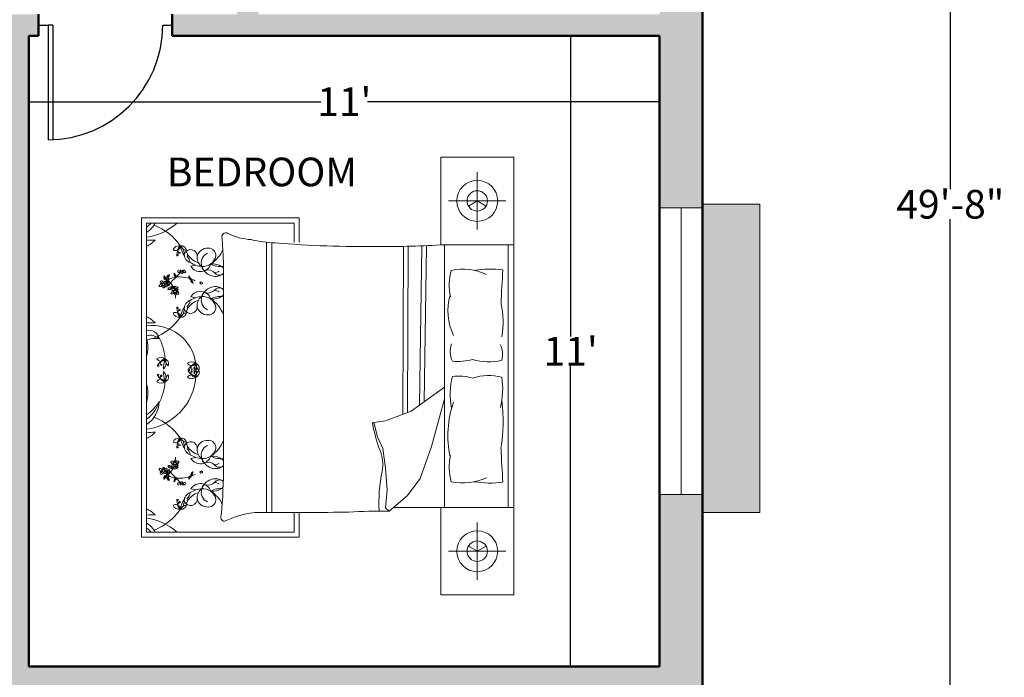
# Model space of a CAD drawing. Units: inches. Extents: x -28 to 544, y -640 to 52.
# Tile 9 of 11: x 338 to 544, y -389 to -251. Entities that reach past the tile are written whole.
import ezdxf

# ---------------------------------------------------------------- set-up
doc = ezdxf.new("R2010")
doc.units = ezdxf.units.IN
doc.header["$MEASUREMENT"] = 0
for name, color, linetype, lineweight in [('A-ANNO-DIMS', 2, 'Continuous', 18), ('A-AREA-IDEN', 7, 'Continuous', 25), ('A-DOOR', 3, 'Continuous', 25), ('A-FURN', 8, 'Continuous', 18), ('A-GLAZ', 4, 'Continuous', 20), ('A-ROOF', 8, 'Continuous', 18), ('A-ROOF-PATT', 252, 'Continuous', 13), ('A-WALL', 7, 'Continuous', 50), ('A-WALL-PATT', 5, 'Continuous', 13)]:
    doc.layers.add(name, color=color, linetype=linetype, lineweight=lineweight)
doc.styles.get("Standard").update_dxf_attribs({"font": 'arial.ttf'})
doc.dimstyles.get("Standard").update_dxf_attribs({"dimtxt": 0.18, "dimasz": 0.18, "dimexe": 0.18, "dimexo": 0.0625, "dimgap": 0.09, "dimtad": 0, "dimtih": 1, "dimtoh": 1, "dimdec": 0, "dimzin": 0, "dimdsep": 46, "dimlunit": 3, "dimtxsty": 'Standard', "dimcen": 0.09, "dimadec": 0, "dimazin": 0, "dimtfac": 1, "dimtdec": 0, "dimtofl": 0, "dimtmove": 0, "dimatfit": 3, "dimfxl": 1, "dimtolj": 1, "dimtzin": 0, "dimarcsym": 0})

# ---------------------------------------------------------------- blocks, each defined once
blk = doc.blocks.new('*D19')
at = {"layer": 'A-ANNO-DIMS', "color": 0, "lineweight": -2, "transparency": 16777216}
for p, q in [((339.44, -274.72), (339.44, -268.35)), ((339.62, -268.53), (400.55, -268.53)), ((471.26, -268.53), (410.34, -268.53)), ((471.44, -274.72), (471.44, -268.35))]:
    blk.add_line(p, q, dxfattribs=at)
at = {"layer": 'A-ANNO-DIMS', "color": 0, "transparency": 16777216}
for points in [[(339.62, -268.5), (339.62, -268.56), (339.44, -268.53)], [(471.26, -268.5), (471.26, -268.56), (471.44, -268.53)]]:
    blk.add_solid(points, dxfattribs=at)
at = {"layer": 'Defpoints', "color": 0, "transparency": 16777216}
for p in [(471.44, -268.53), (339.44, -274.78), (471.44, -274.78)]:
    blk.add_point(p, dxfattribs=at)
at = {"layer": 'A-ANNO-DIMS', "color": 0, "transparency": 16777216, "insert": (405.44, -268.53), "char_height": 6, "attachment_point": 5}
blk.add_mtext("\\A1;11'", dxfattribs=at)
blk = doc.blocks.new('*D20')
at = {"layer": 'A-ANNO-DIMS', "color": 0, "lineweight": -2, "transparency": 16777216}
for p, q in [((452.83, -254.92), (452.83, -317.64)), ((452.89, -254.74), (453.01, -254.74)), ((452.83, -386.56), (452.83, -323.84)), ((452.89, -386.74), (453.01, -386.74))]:
    blk.add_line(p, q, dxfattribs=at)
at = {"layer": 'A-ANNO-DIMS', "color": 0, "transparency": 16777216}
for points in [[(452.8, -254.92), (452.86, -254.92), (452.83, -254.74)], [(452.8, -386.56), (452.86, -386.56), (452.83, -386.74)]]:
    blk.add_solid(points, dxfattribs=at)
at = {"layer": 'Defpoints', "color": 0, "transparency": 16777216}
for p in [(452.83, -254.74), (452.83, -386.74), (452.83, -386.74)]:
    blk.add_point(p, dxfattribs=at)
at = {"layer": 'A-ANNO-DIMS', "color": 0, "transparency": 16777216, "insert": (452.83, -320.74), "char_height": 6, "attachment_point": 5}
blk.add_mtext("\\A1;11'", dxfattribs=at)
blk = doc.blocks.new('*D28')
at = {"layer": 'A-ANNO-DIMS', "color": 0, "lineweight": -2, "transparency": 16777216}
for p, q in [((480.51, 7.76), (532.47, 7.76)), ((532.29, 7.58), (532.29, -286.84)), ((532.29, -587.56), (532.29, -293.14)), ((480.51, -587.74), (532.47, -587.74))]:
    blk.add_line(p, q, dxfattribs=at)
at = {"layer": 'A-ANNO-DIMS', "color": 0, "transparency": 16777216}
for points in [[(532.26, 7.58), (532.32, 7.58), (532.29, 7.76)], [(532.26, -587.56), (532.32, -587.56), (532.29, -587.74)]]:
    blk.add_solid(points, dxfattribs=at)
at = {"layer": 'Defpoints', "color": 0, "transparency": 16777216}
for p in [(480.44, 7.76), (480.44, -587.74), (532.29, -587.74)]:
    blk.add_point(p, dxfattribs=at)
at = {"layer": 'A-ANNO-DIMS', "color": 0, "transparency": 16777216, "insert": (532.29, -289.99), "char_height": 6, "attachment_point": 5}
blk.add_mtext('\\A1;49\'-8"', dxfattribs=at)
blk = doc.blocks.new('BED-DOUBLE-HEADBOARD-92')
for p, q in [((77.93, 0), (77.93, 91.63)), ((70.29, 76.48), (70.29, 88.45)), ((64.3, 82.47), (76.28, 82.47)), ((0, 78.9), (0, 12.09)), ((33.01, 78.9), (0, 78.9)), ((33.01, 73.82), (33.01, 78.9)), ((1.06, 77.84), (31.95, 77.84)), ((1.06, 13.16), (1.06, 77.84)), ((31.95, 77.84), (31.95, 73.8)), ((26.15, 73.81), (26.15, 17.27)), ((27.29, 73.72), (27.29, 17.27)), ((54.87, 72.98), (54.73, 37.82)), ((55.81, 72.98), (55.68, 38.18)), ((58.7, 73.02), (58.23, 39.75)), ((59.64, 73.06), (59.18, 40.44)), ((63.45, 18.33), (63.45, 73.3)), ((76.75, 73.3), (76.75, 18.33)), ((10.35, 68.81), (11.39, 69.01)), ((17.15, 64.42), (17.15, 27.21)), ((10.35, 62.4), (11.39, 62.2)), ((63.45, 43.5), (56.46, 38.48)), ((60.72, 31.05), (63.45, 41.05)), ((56.46, 38.48), (51.08, 36.44)), ((51.08, 36.44), (48.67, 36.07)), ((48.67, 36.07), (49.41, 33.1)), ((49.41, 33.1), (50.52, 30.68)), ((58.31, 24.37), (60.72, 31.05)), ((50.52, 30.68), (51.08, 26.6)), ((10.35, 28.59), (11.39, 28.79)), ((51.08, 26.6), (51.45, 21.96)), ((55.71, 20.85), (58.31, 24.37)), ((10.35, 22.19), (11.39, 21.98)), ((51.45, 21.96), (51.08, 18.25)), ((51.82, 17.51), (55.71, 20.85)), ((31.95, 17.28), (31.95, 13.16)), ((33.01, 12.09), (33.01, 17.28)), ((51.08, 18.25), (51.82, 17.51)), ((77.93, 18.33), (52.78, 18.33)), ((70.29, 15.15), (70.29, 3.18)), ((31.95, 13.16), (1.06, 13.16)), ((0, 12.09), (33.01, 12.09)), ((64.3, 9.16), (76.28, 9.16))]:
    blk.add_line(p, q)
for points in [[(77.93, 73.3), (62.65, 73.3), (62.65, 91.63), (77.93, 91.63)], [(70.29, 82.47), (68.44, 81.4)], [(70.29, 82.47), (72.14, 81.4)], [(62.65, 18.33), (62.65, 0), (77.93, 0)], [(70.29, 9.16), (68.44, 10.23)], [(70.29, 9.16), (72.14, 10.23)]]:
    blk.add_lwpolyline(points)
for points in [[(28.01, 73.7, -0.056112), (22.97, 74.36, -0.095341), (18.12, 75.65)], [(75.64, 68.04, 0.074897), (69.66, 67.93, -0.472817)], [(69.32, 49.3, 0.14099), (75.43, 49.12, 0.235245)], [(69.32, 45.39, -0.14099), (75.43, 45.57, -0.235245)], [(75.64, 23.59, -0.074897), (69.66, 23.7, 0.472817)], [(43.43, 17.31, -0.001242), (26.04, 17.27, 0.127202), (17.38, 15.43)]]:
    blk.add_lwpolyline(points, format="xyb")
for centre, radius in [((70.29, 82.47), 4.28), ((70.29, 82.47), 2.14), ((4.57, 65.04), 0.233), ((7.03, 63.51), 0.233), ((7.03, 27.48), 0.233), ((4.57, 25.95), 0.233), ((70.29, 9.16), 4.28), ((70.29, 9.16), 2.14)]:
    blk.add_circle(centre, radius)
for centre, radius, start, end in [((-2.15, 80.74), 5.83, 303.4617, 330.1116), ((-3.24, 82.84), 7.27, 306.3036, 316.4814), ((-0.55, 86.74), 11.97, 277.745, 311.8856), ((-1.73, 66.27), 11.97, 34.3865, 68.5908), ((-0.8, 77.48), 4.87, 292.5547, 318.9546), ((1.81, 90.8), 16.56, 267.4081, 273.6519), ((17.65, 74.95), 0.835, 56.1736, 203.4781), ((-71.97, 67.22), 89.16, 358.1965, 4.7598), ((7.86, 71.73), 1.33, 77.7115, 159.0387), ((7.14, 73.06), 0.999, 238.4633, 358.2869), ((10.42, 71.04), 3.03, 138.8402, 177.9352), ((8.6, 72.16), 0.979, 117.6827, 223.7762), ((8.38, 72.07), 0.992, 2.9516, 103.728), ((16.31, 74.84), 8.37, 192.5173, 207.1824), ((7.04, 71.5), 1.89, 345.4653, 54.2343), ((9.89, 74.09), 2.04, 211.3827, 255.2969), ((10.28, 70.9), 1.38, 350.264, 160.8688), ((13.81, 70.4), 2.19, 84.9449, 172.8857), ((14.03, 71.03), 1.55, 354.4856, 91.0538), ((10.7, 75.07), 6.94, 303.6671, 336.3547), ((46.26, 287.69), 214.77, 265.1265, 270.8855), ((52.25, 237.57), 164.64, 269.0718, 273.9), ((7.54, 71.14), 0.149, 177.9352, 11.4834), ((7.62, 71.16), 0.0722, 11.4834, 127.9409), ((8.03, 71.59), 0.078, 223.7729, 159.7333), ((10.69, 71.23), 1.72, 175.969, 254.3045), ((8.79, 71.18), 0.843, 333.9755, 53.2681), ((8.41, 69.38), 1.83, 6.1662, 51.5825), ((13.3, 73.63), 4.33, 211.2614, 251.7045), ((14.29, 70.78), 2.66, 182.3591, 234.0401), ((14.64, 69.54), 2.13, 111.5819, 201.4221), ((12.88, 71.51), 2.76, 265.2933, 346.921), ((7.99, 67.72), 0.385, 127.7621, 169.0403), ((8.42, 68.04), 0.233, 183.2768, 356.7232), ((8.78, 67.71), 0.389, 11.5637, 52.6358), ((12.96, 73.67), 4.92, 236.2883, 266.5076), ((12.33, 69.94), 2.28, 209.9085, 343.1337), ((13.28, 68.5), 0.569, 167.3041, 285.1471), ((14.82, 65.78), 3.53, 122.7011, 126.3445), ((15.49, 69.59), 2.92, 199.2822, 299.1751), ((13.92, 66.14), 1.88, 41.5653, 105.1471), ((16.47, 72.53), 3.8, 238.8218, 280.751), ((14.82, 65.78), 3.53, 55.785, 94.7304), ((16.14, 67.83), 1.1, 17.4186, 52.325), ((67.25, 56.37), 11.81, 65.1316, 101.7583), ((947.66, 17.54), 873.48, 176.68521, 177.14978), ((4.91, 66.54), 0.261, 124.3538, 214.3923), ((5.29, 66.5), 0.608, 190.3057, 287.1958), ((5.47, 66.72), 0.705, 176.9701, 248.2913), ((10.5, 70.44), 6.82, 212.6784, 216.3746), ((5.23, 66.56), 0.27, 216.3746, 291.7548), ((3.7, 62.29), 4.06, 63.7819, 68.2913), ((5.88, 66.37), 0.608, 122.8155, 187.3992), ((5.41, 66.12), 0.204, 289.3605, 111.7548), ((5.56, 66.12), 0.204, 221.8703, 44.2646), ((6.14, 66.29), 0.705, 109.4799, 177.6828), ((5.76, 66.74), 0.261, 56.8636, 146.9021), ((5.9, 66.45), 0.27, 148.8844, 224.2646), ((11.5, 63.06), 6.82, 145.1882, 148.8844), ((7.62, 62.77), 3.8, 94.756, 119.2041), ((15.72, 57.29), 12.52, 132.2412, 142.1744), ((9.4, 67.26), 2.58, 178.3264, 187.1302), ((6.61, 66.9), 0.481, 11.3256, 64.4621), ((8.24, 67.59), 1.45, 190.2588, 210.656), ((7.27, 67), 0.44, 188.3432, 274.2869), ((7.66, 67.24), 0.768, 210.656, 242.6341), ((8.24, 67.9), 1.47, 218.2101, 226.3071), ((7.15, 66.67), 0.187, 325.7657, 67.4417), ((1.35, 72.91), 8.7, 313.1541, 322.0459), ((7.81, 58.99), 7.59, 73.5842, 93.8277), ((7.75, 67.68), 0.179, 142.4737, 265.053), ((7.78, 68.04), 0.542, 265.053, 338.3618), ((8.5, 67.3), 0.709, 113.4276, 137.6104), ((8.59, 67.61), 0.382, 139.7889, 227.6792), ((8.47, 67.48), 0.201, 227.6792, 350.3487), ((7.69, 67.62), 0.764, 353.0852, 15.7171), ((8.19, 67.53), 0.482, 350.3487, 43.6538), ((9.08, 68.03), 0.561, 198.7263, 262.5032), ((8.64, 67.76), 0.223, 1.1081, 91.8675), ((9.06, 67.64), 0.18, 255.2356, 54.9248), ((12.48, 66.71), 2.58, 178.3264, 187.1302), ((9.69, 66.35), 0.481, 11.3256, 64.4621), ((11.32, 67.04), 1.45, 190.2588, 210.656), ((10.35, 66.45), 0.44, 188.3432, 274.2869), ((10.74, 66.7), 0.768, 210.656, 242.6341), ((11.32, 67.36), 1.47, 218.2101, 226.3071), ((10.23, 66.12), 0.187, 325.7657, 67.4417), ((10.76, 65.78), 0.44, 147.5332, 233.4768), ((11.15, 66), 0.768, 179.1859, 211.164), ((10.41, 65.83), 0.187, 354.3784, 96.0543), ((7.81, 58.99), 7.59, 63.0032, 69.8941), ((14.96, 70.03), 2.63, 277.436, 299.9149), ((16.35, 68.29), 1.37, 221.5653, 293.8354), ((16.14, 67.83), 1.1, 314.4517, 343.3657), ((76.71, 64.77), 12.28, 165.1039, 191.0369), ((3.9, 64.68), 0.179, 142.4737, 265.053), ((4.14, 64.72), 0.385, 61.2196, 169.0403), ((3.93, 65.05), 0.542, 265.053, 338.3618), ((4.39, 65.51), 0.461, 157.4086, 261.4386), ((4.13, 65.53), 0.231, 58.0499, 135.6268), ((4.65, 64.3), 0.709, 113.4276, 137.6104), ((4.37, 65.38), 0.155, 172.906, 277.132), ((3.87, 65.1), 0.736, 14.7558, 58.0499), ((4.74, 64.62), 0.382, 139.7889, 227.6792), ((4.62, 64.48), 0.201, 227.6792, 350.3487), ((4.9, 65.3), 0.318, 36.1046, 181.4281), ((3.84, 64.62), 0.764, 353.0852, 15.7171), ((4.34, 64.53), 0.482, 350.3487, 43.6538), ((4.71, 65.55), 0.321, 270.0645, 331.1507), ((4.98, 65.47), 0.367, 221.8413, 265.7877), ((5.24, 65.03), 0.561, 198.7263, 262.5032), ((4.79, 64.77), 0.223, 1.1081, 91.8675), ((4.98, 65.33), 0.229, 263.7526, 41.7054), ((4.93, 64.72), 0.389, 11.5637, 86.365), ((7.62, 62.77), 3.8, 124.0033, 132.4917), ((5.21, 64.65), 0.18, 255.2356, 54.9248), ((5.88, 65.42), 0.647, 128.3208, 208.8162), ((5.99, 65.47), 0.773, 207.7043, 254.3516), ((6.48, 65.52), 1.06, 157.2305, 229.0635), ((5.49, 65.02), 1.06, 270.278, 342.111), ((6.2, 63.69), 0.752, 98.7227, 159.3375), ((5.82, 64.66), 0.773, 244.9899, 291.6373), ((6.12, 65.88), 0.626, 174.4544, 220.6188), ((2.56, 62.38), 4.56, 30.544, 49.818), ((5.08, 64.98), 0.752, 340.0041, 40.6188), ((5.99, 65.06), 0.626, 278.7227, 324.8872), ((5.88, 64.55), 0.647, 290.5253, 358.5375), ((6.85, 63.99), 0.461, 157.4086, 261.4386), ((6.59, 64), 0.231, 58.0499, 135.6268), ((7.14, 64.73), 0.647, 182.8499, 266.1226), ((6.89, 65.19), 0.626, 231.7607, 277.9252), ((7.38, 65.3), 1.06, 214.5369, 286.3699), ((6.33, 63.57), 0.736, 14.7558, 58.0499), ((2.56, 62.38), 4.56, 23.0501, 23.8477), ((7.08, 63.82), 0.752, 37.3105, 97.9252), ((7.36, 63.77), 0.318, 36.1046, 181.4281), ((7.16, 64.86), 0.773, 265.0106, 311.658), ((7.44, 63.81), 0.229, 263.7526, 41.7054), ((11.99, 67.54), 2.58, 234.6898, 243.4936), ((11.74, 66.36), 1.45, 211.164, 231.5612), ((12.01, 66.21), 1.47, 195.5129, 203.6099), ((10.35, 65.24), 0.481, 357.3579, 50.4944), ((12.42, 65.34), 0.177, 12.7051, 190.4384), ((12.53, 65.36), 0.287, 190.4384, 10.4136), ((15.49, 61.62), 2.92, 60.8249, 160.7178), ((16.35, 62.91), 1.37, 66.1646, 138.4347), ((16.14, 63.38), 1.1, 23.2856, 45.5483), ((6.36, 63.16), 0.179, 142.4737, 265.053), ((6.6, 63.19), 0.385, 61.2196, 169.0403), ((6.39, 63.52), 0.542, 265.053, 338.3618), ((7.11, 62.78), 0.709, 113.4276, 137.6104), ((6.83, 63.86), 0.155, 172.906, 277.132), ((7.2, 63.09), 0.382, 139.7889, 227.6792), ((7.08, 62.96), 0.201, 227.6792, 350.3487), ((6.3, 63.09), 0.764, 353.0852, 15.7171), ((2.56, 62.38), 4.56, 357.1071, 4.7585), ((6.8, 63), 0.482, 350.3487, 43.6538), ((7.17, 64.02), 0.321, 270.0645, 331.1507), ((7.44, 63.94), 0.367, 221.8413, 265.7877), ((7.7, 63.5), 0.561, 198.7263, 262.5032), ((7.25, 63.24), 0.223, 1.1081, 91.8675), ((7.39, 63.19), 0.389, 11.5637, 86.365), ((7.67, 63.12), 0.18, 255.2356, 54.9248), ((12.96, 57.54), 4.92, 93.4924, 123.7117), ((12.33, 61.27), 2.28, 16.8663, 150.0915), ((14.29, 60.43), 2.66, 125.9599, 177.6409), ((14.64, 61.67), 2.13, 158.5779, 248.4181), ((12.88, 59.7), 2.76, 13.079, 94.7067), ((13.28, 62.71), 0.569, 74.8529, 192.6959), ((14.82, 65.43), 3.53, 233.6555, 237.2989), ((13.92, 65.07), 1.88, 254.8529, 318.4347), ((16.47, 58.68), 3.8, 79.7133, 121.1782), ((14.82, 65.43), 3.53, 265.2696, 304.215), ((10.7, 56.14), 6.94, 21.4941, 56.3329), ((14.96, 61.18), 2.63, 60.0851, 82.564), ((16.14, 63.38), 1.1, 307.675, 336.7144), ((75.81, 59.47), 11.66, 163.8254, 206.1239), ((7.54, 60.07), 0.149, 348.5166, 182.0648), ((10.42, 60.17), 3.03, 182.0648, 221.1598), ((7.62, 60.05), 0.0722, 232.0591, 348.5166), ((7.04, 59.71), 1.89, 305.7657, 14.5347), ((16.31, 56.36), 8.37, 152.8176, 167.4827), ((10.69, 59.98), 1.72, 105.6955, 184.031), ((10.28, 60.31), 1.38, 199.1312, 9.736), ((8.79, 60.02), 0.843, 306.7319, 26.0245), ((8.41, 61.83), 1.83, 308.4175, 353.8338), ((13.3, 57.58), 4.33, 108.2955, 148.7386), ((13.81, 60.81), 2.19, 187.1143, 275.0551), ((14.03, 60.18), 1.55, 268.9462, 5.5144), ((59.61, 57.17), 16.11, 348.8159, 13.6573), ((-0.8, 53.73), 4.87, 41.0454, 67.4453), ((-1.73, 64.94), 11.97, 291.4092, 325.6135), ((7.14, 58.15), 0.999, 1.7131, 121.5367), ((7.86, 59.47), 1.33, 200.9613, 282.2885), ((8.6, 59.04), 0.979, 136.2238, 242.3173), ((7.98, 59.63), 0.129, 200.2817, 136.2238), ((8.38, 59.14), 0.992, 256.272, 357.0484), ((9.89, 57.11), 2.04, 104.7031, 148.6173), ((1.81, 40.41), 16.56, 86.3481, 92.5919), ((2.21, 47.13), 9.26, 8.1803, 97.1364), ((1.57, 53.24), 2.15, 10.9261, 103.6102), ((1.86, 51.63), 2.72, 48.0951, 107.1391), ((-5.23, 51.78), 6.58, 343.5431, 17.0202), ((3.06, 48.33), 5.36, 83.3805, 111.883), ((-6.96, 48.43), 11.97, 4.4623, 27.4146), ((69.49, 50.99), 4.86, 161.4593, 204.9817), ((71.07, 50.37), 4.53, 343.8974, 26.6563), ((-8.62, 49.17), 9.73, 4.3787, 5.6357), ((-15.29, 44.05), 17.39, 19.7217, 19.9028), ((4.08, 48.38), 1.33, 47.7873, 129.1145), ((4.12, 49.89), 0.999, 208.5391, 328.3627), ((3.51, 48.03), 0.149, 148.011, 341.5592), ((5.95, 46.5), 3.03, 108.9159, 148.011), ((3.58, 48), 0.0722, 341.5592, 98.0167), ((4.93, 48.39), 0.979, 87.7585, 193.852), ((4.16, 48.17), 0.078, 193.9791, 129.8091), ((12.96, 46.86), 8.37, 162.593, 177.2582), ((3.25, 48.59), 1.89, 315.5411, 24.3101), ((7.01, 49.42), 2.04, 181.4585, 225.3727), ((4.69, 48.41), 0.992, 333.0274, 73.8037), ((10.49, 47.47), 1.33, 47.7873, 129.1145), ((10.53, 48.97), 0.999, 208.5391, 328.3627), ((12.36, 45.59), 3.03, 108.9159, 148.011), ((11.34, 47.47), 0.979, 87.7585, 193.852), ((9.65, 47.67), 1.89, 315.5411, 24.3101), ((19.37, 45.95), 8.37, 162.593, 177.2582), ((9.65, 46.38), 1.89, 335.6899, 44.4589), ((19.37, 48.1), 8.37, 182.7418, 197.407), ((11.1, 47.5), 0.992, 333.0274, 73.8037), ((13.42, 48.5), 2.04, 181.4585, 225.3727), ((66.26, 60.1), 11.23, 264.0129, 285.8293), ((-0.55, 46.53), 11.97, 277.745, 355.5377), ((3.51, 46.02), 0.149, 18.4408, 211.989), ((5.95, 47.54), 3.03, 211.989, 251.0841), ((3.58, 46.04), 0.0722, 261.9833, 18.4408), ((4.93, 45.66), 0.979, 166.148, 272.2415), ((4.11, 45.86), 0.129, 230.0755, 166.148), ((12.96, 47.19), 8.37, 182.7418, 197.407), ((3.25, 45.46), 1.89, 335.6899, 44.4589), ((7.01, 44.63), 2.04, 134.6273, 178.5415), ((4.69, 45.63), 0.992, 286.1963, 26.9726), ((10.53, 45.07), 0.999, 31.6373, 151.4609), ((10.49, 46.58), 1.33, 230.8855, 312.2127), ((9.92, 47.11), 0.149, 148.011, 341.5592), ((9.92, 46.94), 0.149, 18.4408, 211.989), ((12.36, 48.46), 3.03, 211.989, 251.0841), ((9.99, 47.09), 0.0722, 341.5592, 98.0167), ((9.99, 46.96), 0.0722, 261.9833, 18.4408), ((11.34, 46.58), 0.979, 166.148, 272.2415), ((10.52, 46.78), 0.129, 230.0755, 166.148), ((10.57, 47.26), 0.078, 193.9791, 129.8091), ((11.1, 46.55), 0.992, 286.1963, 26.9726), ((13.42, 45.55), 2.04, 134.6273, 178.5415), ((80.79, 41.94), 16.16, 166.3762, 190.1383), ((66.26, 34.58), 11.23, 74.1707, 95.9871), ((59.28, 43.16), 16.33, 346.04, 8.4751), ((-5.23, 42.27), 6.58, 342.9798, 16.4569), ((-8.62, 44.87), 9.73, 354.3643, 355.6213), ((-15.29, 50), 17.39, 340.0972, 340.2783), ((4.12, 44.16), 0.999, 31.6373, 151.4609), ((4.08, 45.66), 1.33, 230.8855, 312.2127), ((-6.96, 45.61), 11.97, 332.5854, 355.5377), ((-2.15, 40.53), 5.83, 303.4617, 358.728), ((-5.28, 46.44), 10.81, 305.947, 325.9877), ((-3.24, 42.62), 7.27, 306.3036, 342.1496), ((85.44, 33.32), 21.3, 160.7385, 191.9603), ((42.48, 36.14), 33.23, 350.503, 7.7804), ((-1.73, 26.06), 11.97, 34.3865, 68.5908), ((48.59, 35.86), 0.221, 70.2464, 181.1377), ((83.29, 42.43), 35.54, 190.6617, 199.8806), ((1.81, 50.59), 16.56, 267.4081, 273.6519), ((-0.8, 37.26), 4.87, 292.5547, 318.9546), ((7.86, 31.52), 1.33, 77.7115, 159.0387), ((7.14, 32.84), 0.999, 238.4633, 358.2869), ((7.54, 30.93), 0.149, 177.9352, 11.4834), ((10.42, 30.82), 3.03, 138.8402, 177.9352), ((7.62, 30.94), 0.0722, 11.4834, 127.9409), ((8.6, 31.95), 0.979, 117.6827, 223.7762), ((8.03, 31.37), 0.078, 223.7729, 159.7333), ((8.38, 31.85), 0.992, 2.9516, 103.728), ((9.89, 33.88), 2.04, 211.3827, 255.2969), ((7.04, 31.28), 1.89, 345.4653, 54.2343), ((16.31, 34.63), 8.37, 192.5173, 207.1824), ((10.69, 31.02), 1.72, 175.969, 254.3045), ((10.28, 30.69), 1.38, 350.264, 160.8688), ((8.79, 30.97), 0.843, 333.9755, 53.2681), ((13.3, 33.41), 4.33, 211.2614, 251.7045), ((13.81, 30.18), 2.19, 84.9449, 172.8857), ((14.64, 29.32), 2.13, 111.5819, 201.4221), ((14.03, 30.82), 1.55, 354.4856, 91.0538), ((10.7, 34.86), 6.94, 303.6671, 338.5059), ((8.41, 29.17), 1.83, 6.1662, 51.5825), ((12.96, 33.45), 4.92, 236.2883, 266.5076), ((12.33, 29.73), 2.28, 209.9085, 343.1337), ((14.29, 30.56), 2.66, 182.3591, 234.0401), ((12.88, 31.29), 2.76, 265.2933, 346.921), ((16.47, 32.31), 3.8, 238.8218, 280.2867), ((14.82, 25.56), 3.53, 55.785, 94.7304), ((43.05, 27.34), 7.46, 348.6608, 23.7384), ((76.71, 26.86), 12.28, 168.9631, 194.8961), ((947.66, 74.1), 873.48, 182.85022, 183.31479), ((5.82, 26.33), 0.773, 68.3627, 115.0101), ((5.49, 25.97), 1.06, 17.889, 89.722), ((6.2, 27.3), 0.752, 200.6625, 261.2773), ((5.88, 26.45), 0.647, 1.4625, 69.4747), ((6.36, 27.83), 0.179, 94.947, 217.5263), ((6.6, 27.8), 0.385, 190.9597, 298.7804), ((6.39, 27.47), 0.542, 21.6382, 94.947), ((6.85, 27), 0.461, 98.5614, 202.5914), ((6.59, 26.99), 0.231, 224.3732, 301.9501), ((7.14, 26.26), 0.647, 93.8774, 177.1501), ((7.11, 28.21), 0.709, 222.3896, 246.5724), ((6.83, 27.13), 0.155, 82.868, 187.094), ((6.33, 27.42), 0.736, 301.9501, 345.2442), ((2.56, 28.61), 4.56, 336.1523, 336.9499), ((7.2, 27.9), 0.382, 132.3208, 220.2111), ((7.08, 28.04), 0.201, 9.6513, 132.3208), ((6.3, 27.9), 0.764, 344.2829, 6.9148), ((7.36, 27.22), 0.318, 178.5719, 323.8954), ((7.16, 26.14), 0.773, 48.342, 94.9894), ((2.56, 28.61), 4.56, 355.2415, 2.8929), ((6.8, 27.99), 0.482, 316.3462, 9.6513), ((7.7, 27.49), 0.561, 97.4968, 161.2737), ((7.44, 27.05), 0.367, 94.2123, 138.1587), ((7.17, 26.97), 0.321, 28.8493, 89.9355), ((7.25, 27.75), 0.223, 268.1325, 358.8919), ((7.39, 27.8), 0.389, 273.635, 348.4363), ((7.44, 27.19), 0.229, 318.2946, 96.2474), ((7.67, 27.87), 0.18, 305.0752, 104.7644), ((13.28, 28.28), 0.569, 167.3041, 285.1471), ((14.82, 25.56), 3.53, 122.7011, 126.3445), ((15.49, 29.37), 2.92, 199.2822, 299.1751), ((13.92, 25.92), 1.88, 41.5653, 105.1471), ((14.96, 29.81), 2.63, 277.436, 299.9149), ((16.35, 28.08), 1.37, 221.5653, 293.8354), ((-78.23, 26.12), 95.39, 354.3113, 0.6567), ((16.14, 27.61), 1.1, 23.2856, 52.325), ((16.14, 27.61), 1.1, 314.4517, 336.771), ((3.9, 26.31), 0.179, 94.947, 217.5263), ((4.14, 26.27), 0.385, 190.9597, 298.7804), ((3.93, 25.95), 0.542, 21.6382, 94.947), ((4.39, 25.48), 0.461, 98.5614, 202.5914), ((4.13, 25.46), 0.231, 224.3732, 301.9501), ((4.65, 26.69), 0.709, 222.3896, 246.5724), ((4.37, 25.61), 0.155, 82.868, 187.094), ((3.87, 25.89), 0.736, 301.9501, 345.2442), ((4.74, 26.38), 0.382, 132.3208, 220.2111), ((4.62, 26.51), 0.201, 9.6513, 132.3208), ((3.84, 26.37), 0.764, 344.2829, 6.9148), ((4.9, 25.7), 0.318, 178.5719, 323.8954), ((4.34, 26.46), 0.482, 316.3462, 9.6513), ((5.29, 24.49), 0.608, 72.8042, 169.6943), ((5.24, 25.96), 0.561, 97.4968, 161.2737), ((4.98, 25.52), 0.367, 94.2123, 138.1587), ((4.71, 25.45), 0.321, 28.8493, 89.9355), ((5.47, 24.27), 0.705, 111.7087, 183.0299), ((4.79, 26.23), 0.223, 268.1325, 358.8919), ((4.93, 26.28), 0.389, 273.635, 348.4363), ((4.98, 25.66), 0.229, 318.2946, 96.2474), ((7.62, 28.22), 3.8, 227.5083, 235.9967), ((5.21, 26.35), 0.18, 305.0752, 104.7644), ((3.7, 28.7), 4.06, 291.7087, 296.2181), ((5.88, 25.57), 0.647, 151.1838, 231.6792), ((5.99, 25.53), 0.773, 105.6484, 152.2957), ((5.41, 24.88), 0.204, 248.2452, 70.6395), ((5.56, 24.88), 0.204, 315.7354, 138.1297), ((6.48, 25.47), 1.06, 130.9365, 202.7695), ((6.12, 25.12), 0.626, 139.3812, 185.5456), ((2.56, 28.61), 4.56, 310.182, 329.456), ((5.9, 24.55), 0.27, 135.7354, 211.1156), ((5.08, 26.01), 0.752, 319.3812, 19.9959), ((7.62, 28.22), 3.8, 240.7959, 265.244), ((15.72, 33.7), 12.52, 217.8256, 227.7588), ((5.99, 25.94), 0.626, 35.1128, 81.2773), ((7.38, 25.69), 1.06, 73.6301, 145.4631), ((6.89, 25.81), 0.626, 82.0748, 128.2393), ((7.08, 27.17), 0.752, 262.0748, 322.6895), ((10.35, 24.54), 0.44, 85.7131, 171.6568), ((10.74, 24.29), 0.768, 117.3659, 149.344), ((10.23, 24.87), 0.187, 292.5583, 34.2343), ((10.76, 25.21), 0.44, 126.5232, 212.4668), ((11.15, 24.99), 0.768, 148.836, 180.8141), ((10.41, 25.16), 0.187, 263.9457, 5.6216), ((7.81, 32), 7.59, 290.1059, 296.9968), ((11.99, 23.46), 2.58, 116.5064, 125.3102), ((11.74, 24.64), 1.45, 128.4388, 148.836), ((12.01, 24.79), 1.47, 156.3901, 164.4871), ((10.35, 25.75), 0.481, 309.5056, 2.6421), ((12.42, 25.65), 0.177, 169.5616, 347.2949), ((12.53, 25.63), 0.287, 349.5864, 169.5616), ((84.27, 19.07), 34.58, 168.6608, 182.5481), ((4.91, 24.45), 0.261, 145.6077, 235.6462), ((10.5, 20.55), 6.82, 143.6254, 147.3216), ((5.23, 24.44), 0.27, 68.2452, 143.6254), ((5.88, 24.62), 0.608, 172.6008, 237.1845), ((6.14, 24.7), 0.705, 182.3172, 250.5201), ((5.76, 24.26), 0.261, 213.0979, 303.1364), ((11.5, 27.93), 6.82, 211.1156, 214.8118), ((9.4, 23.73), 2.58, 172.8698, 181.6736), ((8.24, 23.4), 1.45, 149.344, 169.7412), ((6.61, 24.09), 0.481, 295.5379, 348.6744), ((7.27, 23.99), 0.44, 85.7131, 171.6568), ((7.66, 23.75), 0.768, 117.3659, 149.344), ((8.24, 23.09), 1.47, 133.6929, 141.7899), ((7.15, 24.33), 0.187, 292.5583, 34.2343), ((7.81, 32), 7.59, 266.1723, 286.4158), ((1.35, 18.08), 8.7, 37.9541, 46.8459), ((7.75, 23.31), 0.179, 94.947, 217.5263), ((7.99, 23.27), 0.385, 190.9597, 232.2379), ((7.78, 22.95), 0.542, 21.6382, 94.947), ((8.5, 23.69), 0.709, 222.3896, 246.5724), ((8.42, 22.96), 0.233, 3.2768, 176.7232), ((8.59, 23.38), 0.382, 132.3208, 220.2111), ((8.47, 23.51), 0.201, 9.6513, 132.3208), ((7.69, 23.37), 0.764, 344.2829, 6.9148), ((8.19, 23.46), 0.482, 316.3462, 9.6513), ((9.08, 22.97), 0.561, 97.4968, 161.2737), ((8.64, 23.23), 0.223, 268.1325, 358.8919), ((9.06, 23.35), 0.18, 305.0752, 104.7644), ((8.78, 23.28), 0.389, 307.3642, 348.4363), ((11.32, 23.95), 1.45, 149.344, 169.7412), ((12.48, 24.28), 2.58, 172.8698, 181.6736), ((9.69, 24.64), 0.481, 295.5379, 348.6744), ((11.32, 23.63), 1.47, 133.6929, 141.7899), ((12.33, 21.05), 2.28, 16.8663, 150.0915), ((13.28, 22.49), 0.569, 74.8529, 192.6959), ((15.49, 21.4), 2.92, 60.8249, 160.7178), ((13.92, 24.86), 1.88, 254.8529, 318.4347), ((14.96, 20.96), 2.63, 60.0851, 82.564), ((16.35, 22.7), 1.37, 66.1646, 138.4347), ((16.14, 23.17), 1.1, 26.442, 45.5483), ((67.25, 35.26), 11.81, 258.2417, 294.8684), ((10.69, 19.76), 1.72, 105.6955, 184.031), ((8.41, 21.61), 1.83, 308.4175, 353.8338), ((13.3, 17.36), 4.33, 108.2955, 148.7386), ((12.96, 17.32), 4.92, 93.4924, 123.7117), ((14.29, 20.21), 2.66, 125.9599, 177.6409), ((14.64, 21.45), 2.13, 158.5779, 248.4181), ((12.88, 19.48), 2.76, 13.079, 94.7067), ((14.82, 25.21), 3.53, 233.6555, 237.2989), ((16.47, 18.46), 3.8, 80.8446, 121.1782), ((14.82, 25.21), 3.53, 265.2696, 304.215), ((10.7, 15.92), 6.94, 26.7003, 56.3329), ((16.14, 23.17), 1.1, 307.675, 329.9707), ((7.14, 17.93), 0.999, 1.7131, 121.5367), ((7.86, 19.26), 1.33, 200.9613, 282.2885), ((7.54, 19.85), 0.149, 348.5166, 182.0648), ((10.42, 19.95), 3.03, 182.0648, 221.1598), ((7.62, 19.83), 0.0722, 232.0591, 348.5166), ((8.6, 18.83), 0.979, 136.2238, 242.3173), ((7.98, 19.42), 0.129, 200.2817, 136.2238), ((16.31, 16.15), 8.37, 152.8176, 167.4827), ((7.04, 19.5), 1.89, 305.7657, 14.5347), ((9.89, 16.9), 2.04, 104.7031, 148.6173), ((8.38, 18.93), 0.992, 256.272, 357.0484), ((10.28, 20.09), 1.38, 199.1312, 9.736), ((8.79, 19.81), 0.843, 306.7319, 26.0245), ((13.81, 20.59), 2.19, 187.1143, 275.0551), ((14.03, 19.96), 1.55, 268.9462, 5.5144), ((-0.8, 13.52), 4.87, 41.0454, 67.4453), ((1.81, 0.19), 16.56, 86.3481, 92.5919), ((-1.73, 24.72), 11.97, 291.4092, 325.6135), ((17.44, 16.28), 0.845, 152.6588, 266.02), ((49.54, -66.51), 84.05, 88.447, 94.1706), ((-0.55, 4.25), 11.97, 48.1144, 82.255), ((-2.15, 10.25), 5.83, 29.8884, 56.5383), ((-3.24, 8.15), 7.27, 43.5186, 53.6964)]:
    blk.add_arc(centre, radius, start, end)
blk = doc.blocks.new('WIN-60IN')
for p, q in [((0, 9), (60, 9)), ((0, 0), (0, 9)), ((60, 9), (60, 0)), ((0, 4.5), (60, 4.5)), ((60, 0), (0, 0))]:
    blk.add_line(p, q)
blk = doc.blocks.new('DOOR-SWING-24IN')
for p, q in [((25, 0), (25, 24)), ((26, 0), (26, 24)), ((2, 0), (0, 0)), ((25, 0), (26, 0)), ((28, 0), (26, 0))]:
    blk.add_line(p, q)
blk.add_arc((26, 0), 24, 90, 180)

msp = doc.modelspace()

# ---------------------------------------------------------------- hatches: boundary and pattern name
at = {"layer": 'A-ROOF-PATT'}
h = msp.add_hatch(color=256, dxfattribs=at)
h.dxf.hatch_style = 1
h.set_gradient(color1=(241, 235, 31), color2=(248, 153, 30))
h.paths.add_polyline_path([(124.53, 19.76), (58.75, 19.76), (58.75, 7.76), (124.53, 7.76)])
h.paths.add_polyline_path([(226.33, 19.76), (182.83, 19.76), (182.83, 7.76), (226.33, 7.76)])
h.paths.add_polyline_path([(313.67, 19.76), (271.84, 19.76), (271.84, 7.76), (313.67, 7.76)])
h.paths.add_polyline_path([(440.55, 19.76), (372.16, 19.76), (372.16, 7.76), (440.55, 7.76)])
h.paths.add_polyline_path([(492.44, -34.91), (480.44, -34.91), (480.44, -100.18), (492.44, -100.18)])
h.paths.add_polyline_path([(492.44, -151.37), (480.44, -151.37), (480.44, -179.02), (492.44, -179.02)])
h.paths.add_polyline_path([(492.44, -207.96), (480.44, -207.96), (480.44, -238.77), (492.44, -238.77)])
h.paths.add_polyline_path([(492.44, -289.99), (480.44, -289.99), (480.44, -354.53), (492.44, -354.53)])
h.paths.add_polyline_path([(492.44, -399.27), (480.44, -399.27), (480.44, -430), (492.44, -430)])
h.paths.add_polyline_path([(492.44, -475.99), (480.44, -475.99), (480.44, -546.14), (492.44, -546.14)])
h.paths.add_polyline_path([(442.7, -587.74), (368.43, -587.74), (368.43, -599.74), (442.7, -599.74)])
h.paths.add_polyline_path([(127.64, -587.74), (54.75, -587.74), (54.75, -599.74), (127.64, -599.74)])
h.paths.add_polyline_path([(16.94, -477.43), (4.94, -477.43), (4.94, -547.54), (16.94, -547.54)])
h.paths.add_polyline_path([(16.94, -399.8), (4.94, -399.8), (4.94, -430.58), (16.94, -430.58)])
h.paths.add_polyline_path([(16.94, -287.93), (4.94, -287.93), (4.94, -356.82), (16.94, -356.82)])
h.paths.add_polyline_path([(16.94, -208.93), (4.94, -208.93), (4.94, -240.18), (16.94, -240.18)])
h.paths.add_polyline_path([(16.94, -150), (4.94, -150), (4.94, -180.17), (16.94, -180.17)])
h.paths.add_polyline_path([(16.94, -32.89), (4.94, -32.89), (4.94, -101.73), (16.94, -101.73)])
at = {"layer": 'A-WALL-PATT'}
h = msp.add_hatch(color=256, dxfattribs=at)
h.dxf.hatch_style = 1
h.paths.add_polyline_path([(375.44, 7.76), (310.94, 7.76), (310.94, -1.24), (334.94, -1.24), (334.94, -133.24), (286.94, -133.24), (286.94, -137.74), (342.44, -137.74), (342.44, -133.24), (339.44, -133.24), (339.44, -1.24), (375.44, -1.24)])
h.paths.add_polyline_path([(480.44, 7.76), (435.44, 7.76), (435.44, -1.24), (471.44, -1.24), (471.44, -37.24), (480.44, -37.24)])
h.paths.add_polyline_path([(480.44, -97.24), (471.44, -97.24), (471.44, -133.24), (417.44, -133.24), (417.44, -135.49), (417.44, -137.74), (471.44, -137.74), (471.44, -152.74), (480.44, -152.74)])
h.paths.add_polyline_path([(480.44, -176.74), (471.44, -176.74), (471.44, -191.74), (387.44, -191.74), (387.44, -137.74), (389.44, -137.74), (389.44, -133.24), (370.44, -133.24), (370.44, -135.49), (370.44, -137.74), (382.94, -137.74), (382.94, -191.74), (382.94, -196.24), (382.94, -220.24), (385.19, -220.24), (387.44, -220.24), (387.44, -196.24), (471.44, -196.24), (471.44, -211.24), (480.44, -211.24)])
h.paths.add_polyline_path([(480.44, -235.24), (471.44, -235.24), (471.44, -250.24), (387.44, -250.24), (387.44, -248.24), (382.94, -248.24), (382.94, -250.24), (369.44, -250.24), (369.44, -252.49), (369.44, -254.74), (471.44, -254.74), (471.44, -290.74), (480.44, -290.74)])
h.paths.add_polyline_path([(480.44, -350.74), (471.44, -350.74), (471.44, -386.74), (339.44, -386.74), (339.44, -254.74), (341.44, -254.74), (341.44, -250.24), (334.94, -250.24), (334.94, -391.24), (471.44, -391.24), (471.44, -403.24), (480.44, -403.24)])
h.paths.add_polyline_path([(480.44, -427.24), (471.44, -427.24), (471.44, -439.24), (334.94, -439.24), (334.94, -446.74), (339.44, -446.74), (339.44, -443.74), (471.44, -443.74), (471.44, -481.24), (480.44, -481.24)])
h.paths.add_polyline_path([(480.44, -541.24), (471.44, -541.24), (471.44, -578.74), (435.44, -578.74), (435.44, -587.74), (480.44, -587.74)])
h.paths.add_polyline_path([(375.44, -578.74), (339.44, -578.74), (339.44, -474.74), (337.19, -474.74), (334.94, -474.74), (334.94, -578.74), (296.69, -578.74), (296.69, -587.74), (375.44, -587.74)])

# ---------------------------------------------------------------- linework, layer by layer
at = {"layer": 'A-ROOF'}
for p, q in [((480.44, -289.99), (492.44, -289.99)), ((492.44, -289.99), (492.44, -354.53)), ((492.44, -354.53), (480.44, -354.53))]:
    msp.add_line(p, q, dxfattribs=at)
at = {"layer": 'A-WALL'}
for p, q in [((480.44, 7.76), (480.44, -587.74)), ((341.44, -254.74), (341.44, -250.24)), ((369.44, -252.49), (369.44, -250.24)), ((369.44, -252.49), (369.44, -254.74)), ((339.44, -254.74), (341.44, -254.74)), ((339.44, -254.74), (339.44, -386.74)), ((369.44, -254.74), (471.44, -254.74)), ((471.44, -254.74), (471.44, -386.74)), ((339.44, -386.74), (471.44, -386.74))]:
    msp.add_line(p, q, dxfattribs=at)

# ---------------------------------------------------------------- block references
at = {"layer": 'A-DOOR', "rotation": 180}
msp.add_blockref('DOOR-SWING-24IN', (369.44, -252.49), dxfattribs=at)
at = {"layer": 'A-FURN'}
msp.add_blockref('BED-DOUBLE-HEADBOARD-92', (362.99, -371.76), dxfattribs=at)
at = {"layer": 'A-GLAZ', "rotation": 90.00000000000003}
msp.add_blockref('WIN-60IN', (480.44, -350.74), dxfattribs=at)

# ---------------------------------------------------------------- texts
at = {"layer": 'A-AREA-IDEN', "insert": (368.3, -280.23), "char_height": 6, "attachment_point": 1}
msp.add_mtext('BEDROOM', dxfattribs=at)

# ---------------------------------------------------------------- dimensions: what is measured, and where the dimension line sits
at = {"layer": 'A-ANNO-DIMS'}
for base, p1, p2, picture, middle in [((532.28608123, -587.74117838), (480.44473605, 7.75882162), (480.44473605, -587.74117838), '*D28', (532.28608123, -289.99117838)), ((452.83, -386.74), (452.83, -254.74), (452.83, -386.74), '*D20', (452.83, -320.74))]:
    dim = msp.add_linear_dim(base=base, p1=p1, p2=p2, angle=90, dimstyle='Standard', override={"dimtxt": 6, "dimclrd": 0, "dimclre": 0, "dimclrt": 0}, dxfattribs=at)
    dim.commit()
    dim.dimension.update_dxf_attribs({"geometry": picture, "text_midpoint": middle})
dim = msp.add_linear_dim(base=(471.44, -268.53), p1=(339.44, -274.78), p2=(471.44, -274.78), dimstyle='Standard', override={"dimtxt": 6, "dimclrd": 0, "dimclre": 0, "dimclrt": 0}, dxfattribs=at)
dim.commit()
dim.dimension.update_dxf_attribs({"geometry": '*D19', "text_midpoint": (405.44, -268.53)})

doc.saveas('drawing.dxf')
